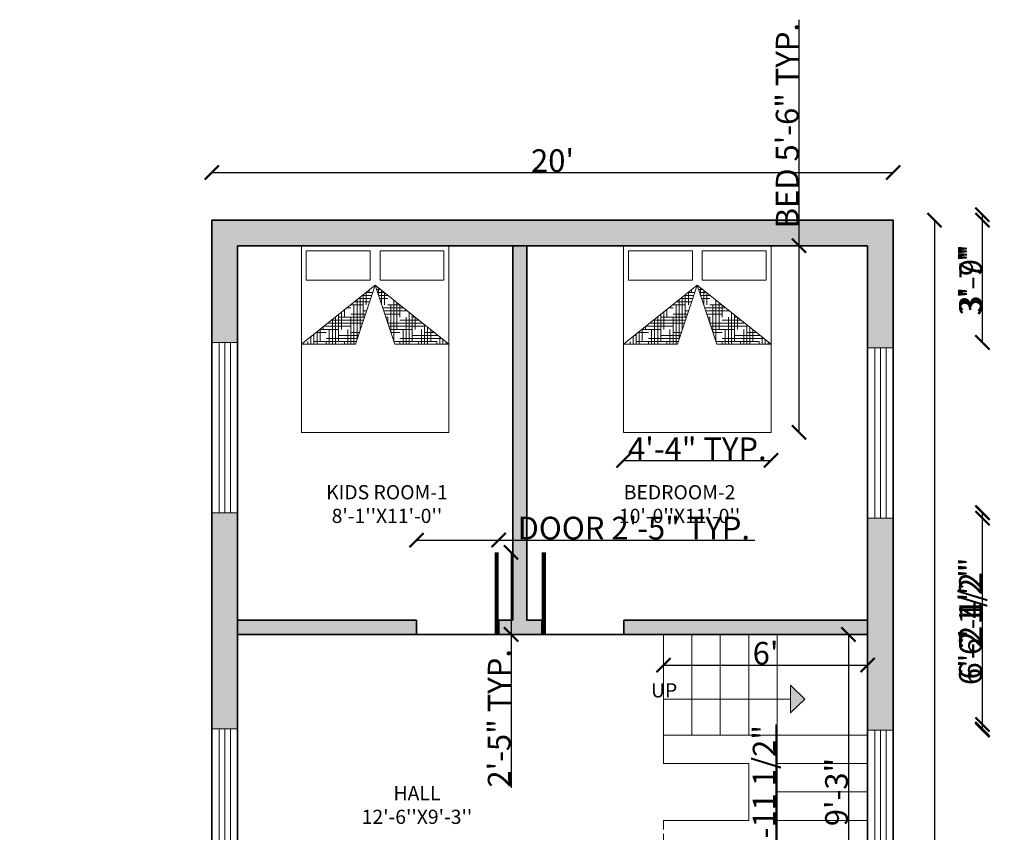
# Model space of a CAD drawing. Units: inches. Extents: x 2267 to 2908, y 1531 to 2136.
# Tile 5 of 5: x 2562 to 2908, y 1849 to 2136. Entities that reach past the tile are written whole.
import ezdxf

# ---------------------------------------------------------------- set-up
doc = ezdxf.new("R2010")
doc.units = ezdxf.units.IN
doc.linetypes.add('HIDDEN', pattern=[9.525, 6.35, -3.175])
for name, color, linetype, lineweight in [('A-ANNO-DIMS', 2, 'Continuous', 18), ('A-ANNO-SYMB', 50, 'Continuous', 18), ('A-ANNO-TEXT', 7, 'Continuous', 18), ('A-AREA-IDEN', 7, 'Continuous', 18), ('A-FLOR-STRS-HIDN', 50, 'HIDDEN', 13), ('A-FURN', 9, 'Continuous', 18), ('A-WALL-PATT', 8, 'Continuous', 13), ('DOOR', 30, 'Continuous', 18), ('STEPS', 50, 'Continuous', 18), ('WALL', 7, 'Continuous', 35), ('WINDOW', 152, 'Continuous', 18)]:
    doc.layers.add(name, color=color, linetype=linetype, lineweight=lineweight)
doc.styles.get("Standard").update_dxf_attribs({"font": 'arial.ttf'})
doc.dimstyles.get("Standard").update_dxf_attribs({"dimtxt": 8, "dimasz": 5, "dimexe": 0.18, "dimexo": 0.0625, "dimgap": 0.09, "dimtad": 1, "dimdec": 1, "dimzin": 0, "dimdsep": 46, "dimlunit": 4, "dimtxsty": 'Standard', "dimblk": 'ARCHTICK', "dimcen": 0.09, "dimse1": 1, "dimse2": 1, "dimadec": 0, "dimazin": 0, "dimtfac": 1, "dimtdec": 1, "dimtofl": 0, "dimtmove": 0, "dimatfit": 3, "dimfxl": 1, "dimtolj": 1, "dimtzin": 0, "dimarcsym": 0})

# ---------------------------------------------------------------- blocks, each defined once
blk = doc.blocks.new('A$C73484D89')
at = {"layer": 'DOOR'}
blk.add_lwpolyline([(1, 0, 0, 0, 0), (1, 0, 0, 0, 0), (0.975, 0, 0.05, 0.05, 0), (0.975, -1, 0, 0, 0), (0.95, -1, 0, 0, -0.429311), (0, 0, 0, 0, 0), (0, 0, 0, 0, 0)], format="xyseb", dxfattribs=at)
blk = doc.blocks.new('*X6')
at = {"color": 0}
for p, q in [((20.156, 14.625), (20.156, 14.728)), ((20.174, 14.75), (20.277, 14.75)), ((20.188, 14.75), (20.188, 14.767)), ((20.199, 14.781), (20.277, 14.781)), ((20.25, 14.812), (20.277, 14.812)), ((20.25, 14.319), (20.25, 14.75)), ((20.094, 14.375), (20.094, 14.65)), ((20.098, 14.656), (20.125, 14.656)), ((20.124, 14.688), (20.25, 14.688)), ((20.125, 14.5), (20.125, 14.689)), ((20.149, 14.719), (20.277, 14.719)), ((19.998, 14.531), (20.277, 14.531)), ((20.023, 14.562), (20.277, 14.562)), ((20.031, 14.247), (20.031, 14.573)), ((20.062, 14.257), (20.062, 14.612)), ((20.125, 14.594), (20.277, 14.594)), ((20.219, 14.309), (20.219, 14.625)), ((20.25, 14.625), (20.277, 14.625)), ((19.922, 14.438), (20, 14.438)), ((19.948, 14.469), (20.125, 14.469)), ((19.973, 14.5), (20.25, 14.5)), ((20, 14.237), (20, 14.5)), ((20.188, 14.299), (20.188, 14.5)), ((20.25, 14.438), (20.277, 14.438)), ((19.844, 14.185), (19.844, 14.34)), ((19.875, 14.25), (19.875, 14.379)), ((19.875, 14.344), (20.277, 14.344)), ((19.906, 14.375), (19.906, 14.417)), ((19.969, 14.226), (19.969, 14.375)), ((20, 14.375), (20.277, 14.375)), ((20.125, 14.406), (20.277, 14.406)), ((20.156, 14.288), (20.156, 14.375)), ((19.772, 14.25), (20, 14.25)), ((19.781, 14.164), (19.781, 14.262)), ((19.797, 14.281), (20.125, 14.281)), ((19.812, 14.174), (19.812, 14.301)), ((19.822, 14.312), (20.229, 14.312)), ((19.938, 14.216), (19.938, 14.25)), ((19.721, 14.188), (19.75, 14.188)), ((19.746, 14.219), (19.875, 14.219)), ((19.75, 14.154), (19.75, 14.223)), ((19.702, 14.094), (19.779, 14.094)), ((19.719, 14.073), (19.719, 14.114)), ((19.727, 14.062), (19.873, 14.062)), ((19.75, 14.034), (19.75, 14.103)), ((19.752, 14.031), (19.875, 14.031)), ((19.781, 13.995), (19.781, 14.093)), ((19.812, 14), (19.812, 14.082)), ((19.906, 13.84), (19.906, 14.051)), ((19.938, 13.801), (19.938, 14.041)), ((19.969, 13.875), (19.969, 14.031)), ((19.827, 13.938), (20.25, 13.938)), ((19.875, 13.878), (19.875, 14)), ((19.875, 13.969), (20.156, 13.969)), ((20, 14), (20, 14.02)), ((20, 14), (20.061, 14)), ((20.062, 13.645), (20.062, 14)), ((20.094, 13.625), (20.094, 13.989)), ((20.125, 13.75), (20.125, 13.979)), ((20.156, 13.875), (20.156, 13.969)), ((20.25, 13.5), (20.25, 13.937)), ((19.853, 13.906), (20.125, 13.906)), ((19.878, 13.875), (20, 13.875)), ((20.031, 13.684), (20.031, 13.875)), ((20.125, 13.844), (20.277, 13.844)), ((20.219, 13.451), (20.219, 13.875)), ((20.25, 13.875), (20.277, 13.875)), ((19.953, 13.781), (20.277, 13.781)), ((19.978, 13.75), (20.25, 13.75)), ((20, 13.812), (20.277, 13.812)), ((20, 13.723), (20, 13.75)), ((20.188, 13.49), (20.188, 13.75)), ((20.003, 13.719), (20.125, 13.719)), ((20.125, 13.656), (20.277, 13.656)), ((20.25, 13.688), (20.277, 13.688)), ((20.079, 13.625), (20.277, 13.625)), ((20.104, 13.594), (20.277, 13.594)), ((20.129, 13.562), (20.25, 13.562)), ((20.156, 13.529), (20.156, 13.625)), ((20.205, 13.469), (20.277, 13.469)), ((20.23, 13.438), (20.277, 13.438)), ((20.25, 13.5), (20.277, 13.5)), ((20.255, 13.406), (20.277, 13.406))]:
    blk.add_line(p, q, dxfattribs=at)
blk = doc.blocks.new('MAT-P13')
for p, q in [((-0.75, 0), (0.75, 0)), ((-0.75, 0), (-0.75, -1.9)), ((0.75, 0), (0.75, -1.9)), ((-0.7, -0.05), (-0.7, -0.35)), ((-0.7, -0.05), (-0.05, -0.05)), ((-0.05, -0.35), (-0.05, -0.05)), ((0.05, -0.05), (0.7, -0.05)), ((0.05, -0.35), (0.05, -0.05)), ((0.7, -0.05), (0.7, -0.35)), ((-0.75, -1.003), (0, -0.4)), ((0, -0.4), (-0.75, -1.003)), ((-0.7, -0.35), (-0.05, -0.35)), ((0, -0.4), (-0.2, -1.003)), ((0, -0.4), (0.2, -1.003)), ((0, -0.4), (0.75, -1.003)), ((0.05, -0.35), (0.7, -0.35)), ((-0.75, -1.003), (-0.2, -1.003)), ((0.2, -1.003), (0.75, -1.003)), ((0.75, -1.9), (-0.75, -1.9))]:
    blk.add_line(p, q)
at = {"xscale": -1, "rotation": 90}
blk.add_blockref('*X6', (14.128, 19.274), dxfattribs=at)
blk = doc.blocks.new('_ArchTick')
at = {"color": 0, "linetype": 'ByBlock', "const_width": 0.15}
blk.add_lwpolyline([(-0.5, -0.5), (0.5, 0.5)], dxfattribs=at)
blk = doc.blocks.new('*D11')
at = {"layer": 'A-ANNO-DIMS', "color": 0, "lineweight": -2, "transparency": 16777216}
blk.add_line((2629.23, 2081.98), (2869.23, 2081.98), dxfattribs=at)
at = {"layer": 'Defpoints', "color": 0, "transparency": 16777216}
for p in [(2869.23, 2081.98), (2629.23, 2065.17), (2869.23, 2065.17)]:
    blk.add_point(p, dxfattribs=at)
at = {"layer": 'A-ANNO-DIMS', "color": 0, "lineweight": -2, "transparency": 16777216, "xscale": 5, "yscale": 5, "zscale": 5, "rotation": 180}
blk.add_blockref('_ArchTick', (2629.23, 2081.98), dxfattribs=at)
at = {"layer": 'A-ANNO-DIMS', "color": 0, "lineweight": -2, "transparency": 16777216, "xscale": 5, "yscale": 5, "zscale": 5}
blk.add_blockref('_ArchTick', (2869.23, 2081.98), dxfattribs=at)
at = {"layer": 'A-ANNO-DIMS', "color": 0, "transparency": 16777216, "insert": (2749.23, 2086.16), "char_height": 8, "attachment_point": 5}
blk.add_mtext("\\A1;20'", dxfattribs=at)
blk = doc.blocks.new('*D12')
at = {"layer": 'A-ANNO-DIMS', "color": 0, "lineweight": -2, "transparency": 16777216}
blk.add_line((2883.79, 2065.17), (2883.79, 1585.17), dxfattribs=at)
at = {"layer": 'Defpoints', "color": 0, "transparency": 16777216}
for p in [(2869.23, 2065.17), (2869.23, 1585.17), (2883.79, 1585.17)]:
    blk.add_point(p, dxfattribs=at)
at = {"layer": 'A-ANNO-DIMS', "color": 0, "lineweight": -2, "transparency": 16777216, "xscale": 5, "yscale": 5, "zscale": 5}
for p, rotation in [((2883.79, 2065.17), 90), ((2883.79, 1585.17), 270)]:
    blk.add_blockref('_ArchTick', p, dxfattribs=dict(at, rotation=rotation))
at = {"layer": 'A-ANNO-DIMS', "color": 0, "transparency": 16777216, "insert": (2879.62, 1825.17), "char_height": 8, "attachment_point": 5, "rotation": 90}
blk.add_mtext("\\A1;40'", dxfattribs=at)
blk = doc.blocks.new('*D13')
at = {"layer": 'A-ANNO-DIMS', "color": 0, "lineweight": -2, "transparency": 16777216}
blk.add_line((2788.33, 1908.4), (2860.23, 1908.4), dxfattribs=at)
at = {"layer": 'Defpoints', "color": 0, "transparency": 16777216}
for p in [(2788.33, 1919.17), (2860.23, 1919.17), (2860.23, 1908.4)]:
    blk.add_point(p, dxfattribs=at)
at = {"layer": 'A-ANNO-DIMS', "color": 0, "lineweight": -2, "transparency": 16777216, "xscale": 5, "yscale": 5, "zscale": 5, "rotation": 180}
blk.add_blockref('_ArchTick', (2788.33, 1908.4), dxfattribs=at)
at = {"layer": 'A-ANNO-DIMS', "color": 0, "lineweight": -2, "transparency": 16777216, "xscale": 5, "yscale": 5, "zscale": 5}
blk.add_blockref('_ArchTick', (2860.23, 1908.4), dxfattribs=at)
at = {"layer": 'A-ANNO-DIMS', "color": 0, "transparency": 16777216, "insert": (2824.28, 1912.57), "char_height": 8, "attachment_point": 5}
blk.add_mtext("\\A1;6'", dxfattribs=at)
blk = doc.blocks.new('*D14')
at = {"layer": 'A-ANNO-DIMS', "color": 0, "lineweight": -2, "transparency": 16777216}
blk.add_line((2853.44, 1919.17), (2853.44, 1808.17), dxfattribs=at)
at = {"layer": 'Defpoints', "color": 0, "transparency": 16777216}
for p in [(2860.23, 1919.17), (2853.44, 1808.17), (2860.23, 1808.17)]:
    blk.add_point(p, dxfattribs=at)
at = {"layer": 'A-ANNO-DIMS', "color": 0, "lineweight": -2, "transparency": 16777216, "xscale": 5, "yscale": 5, "zscale": 5}
for p, rotation in [((2853.44, 1919.17), 90), ((2853.44, 1808.17), 270)]:
    blk.add_blockref('_ArchTick', p, dxfattribs=dict(at, rotation=rotation))
at = {"layer": 'A-ANNO-DIMS', "color": 0, "transparency": 16777216, "insert": (2849.26, 1863.67), "char_height": 8, "attachment_point": 5, "rotation": 90}
blk.add_mtext('\\A1;9\'-3"', dxfattribs=at)
blk = doc.blocks.new('WIN-60IN')
for p, q in [((0, 6.5), (60, 6.5)), ((0, 4.5), (60, 4.5)), ((0, 2.5), (60, 2.5))]:
    blk.add_line(p, q)
blk.add_lwpolyline([(0, 9), (60, 9), (60, 0), (0, 0)], close=True)
blk = doc.blocks.new('WIN-43_65IN')
for p, q in [((2.5, 0), (2.5, 43.65)), ((4.5, 0), (4.5, 43.65)), ((6.5, 0), (6.5, 43.65))]:
    blk.add_line(p, q)
blk.add_lwpolyline([(0, 0), (0, 43.65), (9, 43.65), (9, 0)], close=True)
blk = doc.blocks.new('STAIR-DIRECTION-ARROW')
at = {"transparency": 33554585}
h = blk.add_hatch(color=256, dxfattribs=at)
h.dxf.hatch_style = 1
h.paths.add_polyline_path([(44.76, 9.76), (44.76, 0), (49.76, 4.88)])
for p, q in [((44.76, 9.76), (44.76, 0)), ((49.76, 4.88), (44.76, 9.76)), ((0, 4.88), (44.76, 4.88)), ((49.76, 4.88), (44.76, 0))]:
    blk.add_line(p, q)
blk = doc.blocks.new('*D27')
at = {"layer": 'A-ANNO-DIMS', "color": 0, "lineweight": -2, "transparency": 16777216}
for p, q in [((2701.32, 1952.44), (2730.26, 1952.44)), ((2730.26, 1952.44), (2820.44, 1952.44))]:
    blk.add_line(p, q, dxfattribs=at)
at = {"layer": 'Defpoints', "color": 0, "transparency": 16777216}
for p in [(2730.26, 1952.44), (2701.32, 1948.1), (2730.26, 1948.1)]:
    blk.add_point(p, dxfattribs=at)
at = {"layer": 'A-ANNO-DIMS', "color": 0, "lineweight": -2, "transparency": 16777216, "xscale": 5, "yscale": 5, "zscale": 5, "rotation": 180}
blk.add_blockref('_ArchTick', (2701.32, 1952.44), dxfattribs=at)
at = {"layer": 'A-ANNO-DIMS', "color": 0, "lineweight": -2, "transparency": 16777216, "xscale": 5, "yscale": 5, "zscale": 5}
blk.add_blockref('_ArchTick', (2730.26, 1952.44), dxfattribs=at)
at = {"layer": 'A-ANNO-DIMS', "color": 0, "transparency": 16777216, "insert": (2777.85, 1956.67), "char_height": 8, "attachment_point": 5}
blk.add_mtext('\\A1;DOOR 2\'-5" TYP.', dxfattribs=at)
blk = doc.blocks.new('*D28')
at = {"layer": 'A-ANNO-DIMS', "color": 0, "lineweight": -2, "transparency": 16777216}
for p, q in [((2734.6, 1948.1), (2734.6, 1919.17)), ((2734.6, 1919.17), (2734.6, 1865.09))]:
    blk.add_line(p, q, dxfattribs=at)
at = {"layer": 'Defpoints', "color": 0, "transparency": 16777216}
for p in [(2730.26, 1948.1), (2730.26, 1919.17), (2734.6, 1919.17)]:
    blk.add_point(p, dxfattribs=at)
at = {"layer": 'A-ANNO-DIMS', "color": 0, "lineweight": -2, "transparency": 16777216, "xscale": 5, "yscale": 5, "zscale": 5}
for p, rotation in [((2734.6, 1948.1), 90), ((2734.6, 1919.17), 270)]:
    blk.add_blockref('_ArchTick', p, dxfattribs=dict(at, rotation=rotation))
at = {"layer": 'A-ANNO-DIMS', "color": 0, "transparency": 16777216, "insert": (2730.43, 1889.63), "char_height": 8, "attachment_point": 5, "rotation": 90}
blk.add_mtext('\\A1;2\'-5" TYP.', dxfattribs=at)
blk = doc.blocks.new('*D35')
at = {"layer": 'A-ANNO-DIMS', "color": 0, "lineweight": -2, "transparency": 16777216}
for p, q in [((2828, 1799.95), (2828, 1887.49)), ((2828, 1776.66), (2828, 1799.95))]:
    blk.add_line(p, q, dxfattribs=at)
at = {"layer": 'Defpoints', "color": 0, "transparency": 16777216}
for p in [(2824.51, 1799.95), (2828, 1799.95), (2824.51, 1776.66)]:
    blk.add_point(p, dxfattribs=at)
at = {"layer": 'A-ANNO-DIMS', "color": 0, "lineweight": -2, "transparency": 16777216, "xscale": 5, "yscale": 5, "zscale": 5}
for p, rotation in [((2828, 1799.95), 90), ((2828, 1776.66), 270)]:
    blk.add_blockref('_ArchTick', p, dxfattribs=dict(at, rotation=rotation))
at = {"layer": 'A-ANNO-DIMS', "color": 0, "transparency": 16777216, "insert": (2823.77, 1846.22), "char_height": 8, "attachment_point": 5, "rotation": 90}
blk.add_mtext('\\A1;DOOR 1\'-11 1/2"', dxfattribs=at)
blk = doc.blocks.new('*D47')
at = {"layer": 'A-ANNO-DIMS', "color": 0, "lineweight": -2, "transparency": 16777216}
for p, q in [((2836.06, 2056.17), (2836.06, 2135.85)), ((2836.06, 1990.39), (2836.06, 2056.17))]:
    blk.add_line(p, q, dxfattribs=at)
at = {"layer": 'Defpoints', "color": 0, "transparency": 16777216}
for p in [(2826.19, 2056.17), (2836.06, 2056.17), (2826.19, 1990.39)]:
    blk.add_point(p, dxfattribs=at)
at = {"layer": 'A-ANNO-DIMS', "color": 0, "lineweight": -2, "transparency": 16777216, "xscale": 5, "yscale": 5, "zscale": 5}
for p, rotation in [((2836.06, 2056.17), 90), ((2836.06, 1990.39), 270)]:
    blk.add_blockref('_ArchTick', p, dxfattribs=dict(at, rotation=rotation))
at = {"layer": 'A-ANNO-DIMS', "color": 0, "transparency": 16777216, "insert": (2831.89, 2098.51), "char_height": 8, "attachment_point": 5, "rotation": 90}
blk.add_mtext('\\A1;BED 5\'-6" TYP.', dxfattribs=at)
blk = doc.blocks.new('*D48')
at = {"layer": 'A-ANNO-DIMS', "color": 0, "lineweight": -2, "transparency": 16777216}
blk.add_line((2774.26, 1980.52), (2826.19, 1980.52), dxfattribs=at)
at = {"layer": 'Defpoints', "color": 0, "transparency": 16777216}
for p in [(2774.26, 1990.39), (2826.19, 1990.39), (2826.19, 1980.52)]:
    blk.add_point(p, dxfattribs=at)
at = {"layer": 'A-ANNO-DIMS', "color": 0, "lineweight": -2, "transparency": 16777216, "xscale": 5, "yscale": 5, "zscale": 5, "rotation": 180}
blk.add_blockref('_ArchTick', (2774.26, 1980.52), dxfattribs=at)
at = {"layer": 'A-ANNO-DIMS', "color": 0, "lineweight": -2, "transparency": 16777216, "xscale": 5, "yscale": 5, "zscale": 5}
blk.add_blockref('_ArchTick', (2826.19, 1980.52), dxfattribs=at)
at = {"layer": 'A-ANNO-DIMS', "color": 0, "transparency": 16777216, "insert": (2800.23, 1984.62), "char_height": 8, "attachment_point": 5}
blk.add_mtext('\\A1;4\'-4" TYP.', dxfattribs=at)
blk = doc.blocks.new('*D62')
at = {"layer": 'A-ANNO-DIMS', "color": 0, "lineweight": -2, "transparency": 16777216}
blk.add_line((2900.68, 2022.14), (2900.68, 2067.14), dxfattribs=at)
at = {"layer": 'Defpoints', "color": 0, "transparency": 16777216}
for p in [(2547.81, 2067.14), (2900.68, 2067.14), (2547.81, 2022.14)]:
    blk.add_point(p, dxfattribs=at)
at = {"layer": 'A-ANNO-DIMS', "color": 0, "lineweight": -2, "transparency": 16777216, "xscale": 5, "yscale": 5, "zscale": 5}
for p, rotation in [((2900.68, 2067.14), 90), ((2900.68, 2022.14), 270)]:
    blk.add_blockref('_ArchTick', p, dxfattribs=dict(at, rotation=rotation))
at = {"layer": 'A-ANNO-DIMS', "color": 0, "transparency": 16777216, "insert": (2896.5, 2044.64), "char_height": 8, "attachment_point": 5, "rotation": 90}
blk.add_mtext('\\A1;3\'-9"', dxfattribs=at)
blk = doc.blocks.new('*D63')
at = {"layer": 'A-ANNO-DIMS', "color": 0, "lineweight": -2, "transparency": 16777216}
blk.add_line((2900.68, 2022.08), (2900.68, 2065.17), dxfattribs=at)
at = {"layer": 'Defpoints', "color": 0, "transparency": 16777216}
for p in [(2629.23, 2065.17), (2900.68, 2065.17), (2629.23, 2022.08)]:
    blk.add_point(p, dxfattribs=at)
at = {"layer": 'A-ANNO-DIMS', "color": 0, "lineweight": -2, "transparency": 16777216, "xscale": 5, "yscale": 5, "zscale": 5}
for p, rotation in [((2900.68, 2065.17), 90), ((2900.68, 2022.08), 270)]:
    blk.add_blockref('_ArchTick', p, dxfattribs=dict(at, rotation=rotation))
at = {"layer": 'A-ANNO-DIMS', "color": 0, "transparency": 16777216, "insert": (2896.5, 2043.63), "char_height": 8, "attachment_point": 5, "rotation": 90}
blk.add_mtext('\\A1;3\'-7"', dxfattribs=at)
blk = doc.blocks.new('*D65')
at = {"layer": 'A-ANNO-DIMS', "color": 0, "lineweight": -2, "transparency": 16777216}
blk.add_line((2900.68, 1887.47), (2900.68, 1962.14), dxfattribs=at)
at = {"layer": 'Defpoints', "color": 0, "transparency": 16777216}
for p in [(2547.81, 1962.14), (2900.68, 1962.14), (2547.81, 1887.47)]:
    blk.add_point(p, dxfattribs=at)
at = {"layer": 'A-ANNO-DIMS', "color": 0, "lineweight": -2, "transparency": 16777216, "xscale": 5, "yscale": 5, "zscale": 5}
for p, rotation in [((2900.68, 1962.14), 90), ((2900.68, 1887.47), 270)]:
    blk.add_blockref('_ArchTick', p, dxfattribs=dict(at, rotation=rotation))
at = {"layer": 'A-ANNO-DIMS', "color": 0, "transparency": 16777216, "insert": (2896.45, 1924.8), "char_height": 8, "attachment_point": 5, "rotation": 90}
blk.add_mtext('\\A1;6\'-2 1/2"', dxfattribs=at)
blk = doc.blocks.new('*D67')
at = {"layer": 'A-ANNO-DIMS', "color": 0, "lineweight": -2, "transparency": 16777216}
blk.add_line((2900.68, 1885.88), (2900.68, 1962.08), dxfattribs=at)
at = {"layer": 'Defpoints', "color": 0, "transparency": 16777216}
for p in [(2629.23, 1962.08), (2900.68, 1962.08), (2629.23, 1885.88)]:
    blk.add_point(p, dxfattribs=at)
at = {"layer": 'A-ANNO-DIMS', "color": 0, "lineweight": -2, "transparency": 16777216, "xscale": 5, "yscale": 5, "zscale": 5}
for p, rotation in [((2900.68, 1962.08), 90), ((2900.68, 1885.88), 270)]:
    blk.add_blockref('_ArchTick', p, dxfattribs=dict(at, rotation=rotation))
at = {"layer": 'A-ANNO-DIMS', "color": 0, "transparency": 16777216, "insert": (2896.5, 1923.98), "char_height": 8, "attachment_point": 5, "rotation": 90}
blk.add_mtext('\\A1;6\'-4"', dxfattribs=at)
blk = doc.blocks.new('*D71')
at = {"layer": 'A-ANNO-DIMS', "color": 0, "lineweight": -2, "transparency": 16777216}
blk.add_line((2900.68, 1885.5), (2900.68, 1960.17), dxfattribs=at)
at = {"layer": 'Defpoints', "color": 0, "transparency": 16777216}
for p in [(2869.23, 1960.17), (2900.68, 1960.17), (2869.23, 1885.5)]:
    blk.add_point(p, dxfattribs=at)
at = {"layer": 'A-ANNO-DIMS', "color": 0, "lineweight": -2, "transparency": 16777216, "xscale": 5, "yscale": 5, "zscale": 5}
for p, rotation in [((2900.68, 1960.17), 90), ((2900.68, 1885.5), 270)]:
    blk.add_blockref('_ArchTick', p, dxfattribs=dict(at, rotation=rotation))
at = {"layer": 'A-ANNO-DIMS', "color": 0, "transparency": 16777216, "insert": (2896.45, 1922.83), "char_height": 8, "attachment_point": 5, "rotation": 90}
blk.add_mtext('\\A1;6\'-2 1/2"', dxfattribs=at)

msp = doc.modelspace()

# ---------------------------------------------------------------- hatches: boundary and pattern name
at = {"layer": 'A-WALL-PATT', "transparency": 33554585}
h = msp.add_hatch(color=256, dxfattribs=at)
h.dxf.hatch_style = 1
h.paths.add_polyline_path([(2547.81, 2067.14), (2395.31, 2067.14), (2395.31, 2058.14), (2413.81, 2058.14), (2538.81, 2058.14), (2538.81, 2022.14), (2547.81, 2022.14)])
h.paths.add_polyline_path([(2335.31, 2067.14), (2307.81, 2067.14), (2307.81, 1992.99), (2316.81, 1992.99), (2316.81, 2058.14), (2335.31, 2058.14)])
h.paths.add_polyline_path([(2316.81, 1949.34), (2307.81, 1949.34), (2307.81, 1886.58), (2316.81, 1886.58)])
h.paths.add_polyline_path([(2316.81, 1842.93), (2307.81, 1842.93), (2307.81, 1791.76), (2316.81, 1791.76)])
h.paths.add_polyline_path([(2316.81, 1769.93), (2307.81, 1769.93), (2307.81, 1695.97), (2316.81, 1695.97)])
h.paths.add_polyline_path([(2316.81, 1652.32), (2307.81, 1652.32), (2307.81, 1587.14), (2344.81, 1587.14), (2344.81, 1596.14), (2316.81, 1596.14)])
h.paths.add_polyline_path([(2441.81, 1715.23, -0.025641), (2438.4, 1715.23), (2436.81, 1715.23), (2436.81, 1596.14), (2404.81, 1596.14), (2404.81, 1587.14), (2441.81, 1587.14)])
h.paths.add_polyline_path([(2547.81, 1770.23), (2538.81, 1770.23), (2538.81, 1752.14), (2542.81, 1752.14), (2542.81, 1587.14), (2547.81, 1587.14)])
h.paths.add_polyline_path([(2547.81, 1843.82), (2538.81, 1843.82), (2538.81, 1792.05), (2547.81, 1792.05)])
h.paths.add_polyline_path([(2547.81, 1962.14), (2538.81, 1962.14), (2538.81, 1887.47), (2547.81, 1887.47)])
h.paths.add_polyline_path([(2638.23, 1962.08), (2629.23, 1962.08), (2629.23, 1885.88), (2638.23, 1885.88)])
h.paths.add_polyline_path([(2638.23, 2056.17), (2860.23, 2056.17), (2860.23, 2020.17), (2869.23, 2020.17), (2869.23, 2065.17), (2629.23, 2065.17), (2629.23, 2022.08), (2638.23, 2022.08)])
h.paths.add_polyline_path([(2869.23, 1960.17), (2860.23, 1960.17), (2860.23, 1885.5), (2869.23, 1885.5)])
h.paths.add_polyline_path([(2869.23, 1841.85), (2860.23, 1841.85), (2860.23, 1790.08), (2869.23, 1790.08)])
h.paths.add_polyline_path([(2869.23, 1768.26), (2860.23, 1768.26), (2860.23, 1768.05), (2860.23, 1720.44), (2869.23, 1720.44)])
h.paths.add_polyline_path([(2869.23, 1660.44), (2860.23, 1660.44), (2860.23, 1585.17), (2869.23, 1585.17)])
h.paths.add_polyline_path([(2763.23, 1594.17), (2726.23, 1594.17), (2726.23, 1585.17), (2763.23, 1585.17)])
h.paths.add_polyline_path([(2666.23, 1594.17), (2638.23, 1594.17), (2638.23, 1768.3), (2629.23, 1768.3), (2629.23, 1585.17), (2666.23, 1585.17)])
h.paths.add_polyline_path([(2638.23, 1842.24), (2629.23, 1842.24), (2629.23, 1790.12), (2638.23, 1790.12)])
h = msp.add_hatch(color=256, dxfattribs=at)
h.dxf.hatch_style = 1
h.paths.add_polyline_path([(2763.23, 1755.17), (2758.23, 1755.17), (2758.23, 1625.17), (2760.21, 1625.17, -0.025641), (2763.23, 1625.17)])
h.paths.add_polyline_path([(2638.23, 1750.17), (2679.86, 1750.17, -0.025641), (2679.86, 1752.99), (2679.86, 1755.17), (2638.23, 1755.17)])
h.paths.add_polyline_path([(2860.23, 1625.17), (2860.23, 1630.17), (2796.25, 1630.17), (2796.25, 1628.39, -0.025641), (2796.25, 1625.17)])
h.paths.add_polyline_path([(2730.26, 1919.17), (2745.45, 1919.17), (2745.45, 1924.17), (2740.23, 1924.17), (2740.23, 2056.17), (2735.23, 2056.17), (2735.23, 1924.17), (2730.26, 1924.17)])
h.paths.add_polyline_path([(2860.23, 1919.17), (2860.23, 1924.17), (2774.38, 1924.17), (2774.38, 1921.99, -0.025641), (2774.38, 1919.17)])
h.paths.add_polyline_path([(2638.23, 1919.17), (2701.33, 1919.17, -0.025641), (2701.33, 1921.99), (2701.33, 1924.17), (2638.23, 1924.17)])
h.paths.add_polyline_path([(2538.81, 1752.14), (2538.81, 1757.14), (2441.81, 1757.14), (2441.81, 1762.09), (2439.73, 1762.09, -0.025641), (2436.81, 1762.09), (2436.81, 1750.17), (2441.81, 1750.17), (2441.81, 1752.14)])
h.paths.add_polyline_path([(2436.81, 1810.14), (2436.81, 1792.08), (2441.81, 1792.08), (2441.81, 1805.14), (2538.81, 1805.14), (2538.81, 1810.14)])
h.paths.add_polyline_path([(2346.81, 1805.14), (2346.81, 1810.14), (2316.81, 1810.14), (2316.81, 1805.14)], flags=0)
h.paths.add_polyline_path([(2376.81, 1810.14), (2371.81, 1810.14), (2371.81, 1757.14), (2316.81, 1757.14), (2316.81, 1752.14), (2376.81, 1752.14)])
h.paths.add_polyline_path([(2374.47, 1921.14), (2374.47, 1926.14), (2316.81, 1926.14), (2316.81, 1921.14)])
h.paths.add_polyline_path([(2413.81, 1921.14), (2421.94, 1921.14), (2421.94, 1926.14), (2418.81, 1926.14), (2418.81, 2058.14), (2413.81, 2058.14)])
h.paths.add_polyline_path([(2316.81, 2022.14), (2316.81, 2017.14), (2381.27, 2017.14), (2381.27, 2022.14)])
h.paths.add_polyline_path([(2455.63, 1926.14), (2455.63, 1924.43, -0.025641), (2455.63, 1921.14), (2538.81, 1921.14), (2538.81, 1926.14)])

# ---------------------------------------------------------------- linework, layer by layer
at = {"layer": 'A-FLOR-STRS-HIDN', "ltscale": 0.5}
msp.add_line((2788.33, 1853.67), (2788.33, 1808.17), dxfattribs=at)
at = {"layer": 'STEPS'}
for p, q in [((2788.33, 1919.17), (2788.33, 1873.67)), ((2798.33, 1919.17), (2798.33, 1883.67)), ((2808.33, 1919.17), (2808.33, 1883.67)), ((2818.33, 1919.17), (2818.33, 1883.67)), ((2828.33, 1919.17), (2828.33, 1843.67)), ((2788.33, 1883.67), (2860.23, 1883.67)), ((2788.33, 1873.67), (2818.33, 1873.67)), ((2818.33, 1873.67), (2818.33, 1853.67)), ((2828.33, 1873.67), (2860.33, 1873.67)), ((2828.33, 1863.67), (2860.23, 1863.67)), ((2818.33, 1853.67), (2788.33, 1853.67)), ((2828.33, 1853.67), (2860.23, 1853.67))]:
    msp.add_line(p, q, dxfattribs=at)
at = {"layer": 'WALL'}
for p, q in [((2629.23, 2065.17), (2869.23, 2065.17)), ((2629.23, 2065.17), (2629.23, 1585.17)), ((2869.23, 2065.17), (2869.23, 1585.17)), ((2638.23, 2056.17), (2860.23, 2056.17)), ((2638.23, 2056.17), (2638.23, 1594.17)), ((2735.23, 2056.17), (2735.23, 1924.17)), ((2740.23, 2056.17), (2740.23, 1924.17)), ((2860.23, 2056.17), (2860.23, 1585.17)), ((2638.23, 1924.17), (2701.33, 1924.17)), ((2701.33, 1924.17), (2701.33, 1921.99)), ((2701.33, 1921.99), (2701.33, 1919.17)), ((2730.26, 1924.17), (2730.26, 1919.17)), ((2730.26, 1924.17), (2735.23, 1924.17)), ((2740.23, 1924.17), (2745.45, 1924.17)), ((2745.45, 1924.17), (2745.45, 1919.17)), ((2774.38, 1924.17), (2774.38, 1921.99)), ((2774.38, 1924.17), (2860.23, 1924.17)), ((2774.38, 1921.99), (2774.38, 1919.17)), ((2638.23, 1919.17), (2860.23, 1919.17))]:
    msp.add_line(p, q, dxfattribs=at)

# ---------------------------------------------------------------- block references
at = {"layer": 'A-ANNO-SYMB'}
msp.add_blockref('STAIR-DIRECTION-ARROW', (2788.33, 1891.54), dxfattribs=at)
at = {"layer": 'A-FURN', "xscale": 34.62184577987068, "yscale": 34.62184577987068, "zscale": 34.62184577987068}
for p in [(2686.73, 2056.17), (2800.23, 2056.17)]:
    msp.add_blockref('MAT-P13', p, dxfattribs=at)
at = {"layer": 'DOOR', "yscale": 28.92760358030192, "zscale": 28.92760358030192, "rotation": 180}
for p, xscale in [((2701.33, 1919.17), -28.92760358030192), ((2774.38, 1919.17), 28.92760358030192)]:
    msp.add_blockref('A$C73484D89', p, dxfattribs=dict(at, xscale=xscale))
at = {"layer": 'WINDOW'}
for p, rotation in [((2638.23, 1962.08), 89.99999999999876), ((2869.23, 1960.17), 89.9999999999986)]:
    msp.add_blockref('WIN-60IN', p, dxfattribs=dict(at, rotation=rotation))
for p in [(2629.23, 1842.24), (2860.23, 1841.85)]:
    msp.add_blockref('WIN-43_65IN', p, dxfattribs=at)

# ---------------------------------------------------------------- texts
at = {"layer": 'A-ANNO-TEXT', "insert": (2767.84, 1902), "char_height": 5, "attachment_point": 1}
msp.add_mtext_dynamic_manual_height_columns('\\pxqc;UP', width=41.4104, gutter_width=12.5, heights=[0], dxfattribs=at)
at = {"layer": 'A-AREA-IDEN', "char_height": 5, "attachment_point": 1}
for s, width, insert in [("\\pxqc;KIDS ROOM-1\\P8'-1''X11'-0''", 53.0678, (2664.36, 1971.81)), ("\\pxqc;BEDROOM-2\\P10'-0''X11'-0''", 41.4104, (2773.28, 1971.81)), ("\\pxqc;HALL\\P12'-6''X9'-3''", 41.4104, (2680.76, 1865.75))]:
    msp.add_mtext_dynamic_manual_height_columns(s, width=width, gutter_width=12.5, heights=[0], dxfattribs=dict(at, insert=insert))

# ---------------------------------------------------------------- dimensions: what is measured, and where the dimension line sits
at = {"layer": 'A-ANNO-DIMS'}
for base, p1, p2, angle, text, picture, middle in [((2836.06, 2056.17), (2826.19, 1990.39), (2826.19, 2056.17), 90, 'BED <> TYP.', '*D47', (2831.89, 2098.51)), ((2734.6, 1919.17), (2730.26, 1948.1), (2730.26, 1919.17), 270, '<> TYP.', '*D28', (2730.43, 1889.63)), ((2828, 1799.95), (2824.51, 1776.66), (2824.51, 1799.95), 90, 'DOOR <>', '*D35', (2823.77, 1846.22))]:
    dim = msp.add_linear_dim(base=base, p1=p1, p2=p2, angle=angle, text=text, dimstyle='Standard', override={"dimdec": 1, "dimlfac": 1, "dimrnd": 0, "dimzin": 1, "dimdsep": 46, "dimlunit": 4, "dimfrac": 2}, dxfattribs=at)
    dim.commit()
    dim.dimension.update_dxf_attribs({"geometry": picture, "text_midpoint": middle})
for base, p1, p2, picture, middle in [((2869.23, 2081.98), (2629.23, 2065.17), (2869.23, 2065.17), '*D11', (2749.23, 2086.16)), ((2860.23, 1908.4), (2788.33, 1919.17), (2860.23, 1919.17), '*D13', (2824.28, 1912.57))]:
    dim = msp.add_linear_dim(base=base, p1=p1, p2=p2, dimstyle='Standard', override={"dimclrd": 0, "dimclre": 0, "dimclrt": 0}, dxfattribs=at)
    dim.commit()
    dim.dimension.update_dxf_attribs({"geometry": picture, "text_midpoint": middle})
for base, p1, p2, override, picture, middle in [((2900.68, 2067.14), (2547.81, 2022.14), (2547.81, 2067.14), {"dimdec": 1, "dimlfac": 1, "dimrnd": 0, "dimzin": 1, "dimdsep": 46, "dimlunit": 4, "dimfrac": 2}, '*D62', (2896.5, 2044.64)), ((2900.68, 2065.17), (2629.23, 2022.08), (2629.23, 2065.17), {"dimdec": 1, "dimlfac": 1, "dimrnd": 0, "dimzin": 1, "dimdsep": 46, "dimlunit": 4, "dimfrac": 2}, '*D63', (2896.5, 2043.63)), ((2883.79, 1585.17), (2869.23, 2065.17), (2869.23, 1585.17), {"dimclrd": 0, "dimclre": 0, "dimclrt": 0}, '*D12', (2879.62, 1825.17)), ((2900.68, 1962.14), (2547.81, 1887.47), (2547.81, 1962.14), {"dimdec": 1, "dimlfac": 1, "dimrnd": 0, "dimzin": 1, "dimdsep": 46, "dimlunit": 4, "dimfrac": 2}, '*D65', (2896.45, 1924.8)), ((2900.68, 1962.08), (2629.23, 1885.88), (2629.23, 1962.08), {"dimdec": 1, "dimlfac": 1, "dimrnd": 0, "dimzin": 1, "dimdsep": 46, "dimlunit": 4, "dimfrac": 2}, '*D67', (2896.5, 1923.98)), ((2900.68, 1960.17), (2869.23, 1885.5), (2869.23, 1960.17), {"dimdec": 1, "dimlfac": 1, "dimrnd": 0, "dimzin": 1, "dimdsep": 46, "dimlunit": 4, "dimfrac": 2}, '*D71', (2896.45, 1922.83)), ((2853.44, 1808.17), (2860.23, 1919.17), (2860.23, 1808.17), {"dimclrd": 0, "dimclre": 0, "dimclrt": 0}, '*D14', (2849.26, 1863.67))]:
    dim = msp.add_linear_dim(base=base, p1=p1, p2=p2, angle=90, dimstyle='Standard', override=override, dxfattribs=at)
    dim.commit()
    dim.dimension.update_dxf_attribs({"geometry": picture, "text_midpoint": middle})
for base, p1, p2, text, picture, middle in [((2826.19, 1980.52), (2774.26, 1990.39), (2826.19, 1990.39), '<> TYP.', '*D48', (2800.23, 1984.62)), ((2730.26, 1952.44), (2701.32, 1948.1), (2730.26, 1948.1), 'DOOR <> TYP.', '*D27', (2777.85, 1956.67))]:
    dim = msp.add_linear_dim(base=base, p1=p1, p2=p2, text=text, dimstyle='Standard', override={"dimdec": 1, "dimlfac": 1, "dimrnd": 0, "dimzin": 1, "dimdsep": 46, "dimlunit": 4, "dimfrac": 2}, dxfattribs=at)
    dim.commit()
    dim.dimension.update_dxf_attribs({"geometry": picture, "text_midpoint": middle})

doc.saveas('drawing.dxf')
